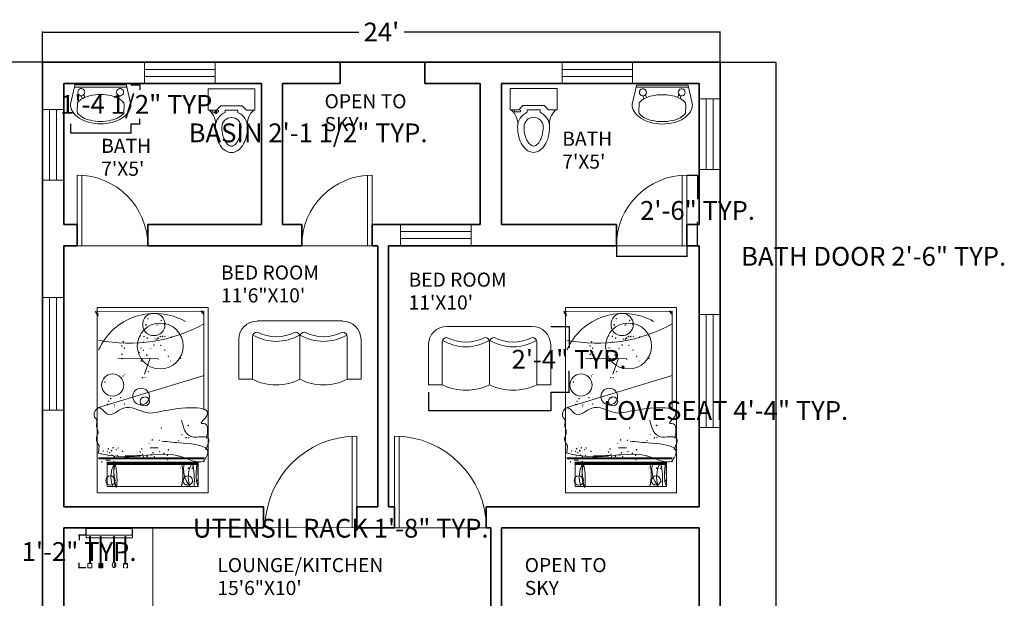
# Model space of a CAD drawing. Units: inches. Extents: x 125 to 976, y 231 to 853.
# Tile 16 of 16: x 557 to 976, y 584 to 830. Entities that reach past the tile are written whole.
import ezdxf

# ---------------------------------------------------------------- set-up
doc = ezdxf.new("R2010")
doc.units = ezdxf.units.IN
doc.header["$MEASUREMENT"] = 0
for name, color, linetype, lineweight in [('A-ANNO-DIMS', 2, 'Continuous', 18), ('A-AREA-IDEN', 7, 'Continuous', 18), ('A-DOOR', 3, 'Continuous', 18), ('A-EQPM', 8, 'Continuous', 15), ('A-FLOR-CASE', 32, 'Continuous', 18), ('A-FLOR-FIXT', 9, 'Continuous', 18), ('A-GLAZ', 4, 'Continuous', 18), ('A-WALL', 7, 'Continuous', 35), ('Furniture', 8, 'Continuous', 15)]:
    doc.layers.add(name, color=color, linetype=linetype, lineweight=lineweight)
doc.styles.get("Standard").update_dxf_attribs({"font": 'italic8.shx'})
doc.dimstyles.get("Standard").update_dxf_attribs({"dimtxt": 8, "dimasz": 0.18, "dimexe": 0.18, "dimexo": 0.0625, "dimgap": 0.09, "dimtad": 0, "dimtih": 1, "dimtoh": 1, "dimdec": 4, "dimzin": 0, "dimdsep": 46, "dimlunit": 3, "dimtxsty": 'Standard', "dimcen": 0.09, "dimclrt": 4, "dimadec": 0, "dimazin": 0, "dimtfac": 1, "dimtdec": 4, "dimtofl": 0, "dimtmove": 0, "dimatfit": 3, "dimfxl": 1, "dimtolj": 1, "dimtzin": 0, "dimarcsym": 0})

# ---------------------------------------------------------------- blocks, each defined once
blk = doc.blocks.new('*D5')
at = {"layer": 'A-ANNO-DIMS', "color": 0, "lineweight": -2, "transparency": 16777216}
for p, q in [((567.19, 812.17), (567.19, 825.16)), ((567.37, 824.98), (701.58, 824.98)), ((855.01, 824.98), (720.81, 824.98)), ((855.19, 812.17), (855.19, 825.16))]:
    blk.add_line(p, q, dxfattribs=at)
at = {"layer": 'A-ANNO-DIMS', "color": 0, "transparency": 16777216}
for points in [[(567.37, 825.01), (567.37, 824.95), (567.19, 824.98)], [(855.01, 825.01), (855.01, 824.95), (855.19, 824.98)]]:
    blk.add_solid(points, dxfattribs=at)
at = {"layer": 'Defpoints', "color": 0, "transparency": 16777216}
for p in [(855.19, 824.98), (567.19, 812.1), (855.19, 812.1)]:
    blk.add_point(p, dxfattribs=at)
at = {"layer": 'A-ANNO-DIMS', "color": 0, "transparency": 16777216, "insert": (711.19, 824.98), "char_height": 8, "attachment_point": 5}
blk.add_mtext("\\A1;24'", dxfattribs=at)
blk = doc.blocks.new('*D6')
at = {"layer": 'A-ANNO-DIMS', "color": 0, "lineweight": -2, "transparency": 16777216}
for p, q in [((855.26, 812.1), (878.96, 812.1)), ((878.78, 811.92), (878.78, 546.96)), ((878.78, 272.28), (878.78, 537.25)), ((846.26, 272.1), (878.96, 272.1))]:
    blk.add_line(p, q, dxfattribs=at)
at = {"layer": 'A-ANNO-DIMS', "color": 0, "transparency": 16777216}
for points in [[(878.75, 811.92), (878.81, 811.92), (878.78, 812.1)], [(878.75, 272.28), (878.81, 272.28), (878.78, 272.1)]]:
    blk.add_solid(points, dxfattribs=at)
at = {"layer": 'Defpoints', "color": 0, "transparency": 16777216}
for p in [(855.19, 812.1), (846.19, 272.1), (878.78, 272.1)]:
    blk.add_point(p, dxfattribs=at)
at = {"layer": 'A-ANNO-DIMS', "color": 0, "transparency": 16777216, "insert": (878.78, 542.1), "char_height": 8, "attachment_point": 5}
blk.add_mtext("\\A1;45'", dxfattribs=at)
blk = doc.blocks.new('BED-SINGLE')
for p, q in [((45.57, 77.25), (0.68, 77.02)), ((1.36, 0), (1.36, 78.74)), ((1.36, 78.74), (48.6, 78.74)), ((46.62, 76.32), (45.83, 76.32)), ((46.75, 35.25), (46.75, 77.26)), ((48.6, 78.74), (48.6, 0)), ((46.75, 35.25), (46.75, 75.28)), ((10.09, 57.07), (27.33, 57.29)), ((21.53, 50.36), (23.91, 57.3)), ((46.77, 49.81), (2, 36.21)), ((46.74, 50.11), (46.74, 35.53)), ((2.2, 19.89), (1.98, 16.84)), ((23.9, 19.06), (27.33, 19.06)), ((46.77, 14.92), (2, 14.9)), ((46.77, 14.62), (2, 14.6)), ((46.75, 14.47), (2.3, 14.45)), ((5.12, 13.84), (6.96, 13.84)), ((44.11, 12.79), (5.52, 12.79)), ((44.11, 12.66), (5.52, 12.66)), ((5.56, 2.64), (5.56, 12.97)), ((5.56, 12.97), (44.32, 12.97)), ((44.26, 2.65), (44.11, 12.79)), ((44.32, 12.97), (44.32, 2.64)), ((44.11, 12.36), (5.52, 12.36)), ((44.11, 12.07), (5.52, 12.07)), ((44.32, 2.64), (5.56, 2.64)), ((1.36, 0), (48.6, 0))]:
    blk.add_line(p, q)
for centre, radius in [((25.44, 71.55), 4.72), ((28.17, 62.4), 9.76), ((22.09, 71.4), 0.118), ((22.93, 74.08), 0.0787), ((26.78, 71.35), 0.118), ((27.34, 71.86), 0.0394), ((28.65, 73.29), 0.118), ((30.02, 71.69), 0.118), ((12.45, 64.21), 0.118), ((19.72, 66.71), 0.118), ((21.26, 66.47), 0.118), ((21.3, 64.04), 0.0787), ((22.64, 65.78), 0.118), ((25.46, 62.84), 0.118), ((25.97, 65.38), 0.0394), ((26.83, 65.34), 0.118), ((27.33, 65.73), 0.118), ((28.16, 66.42), 0.118), ((29.11, 66.45), 0.118), ((30.23, 66.51), 0.0787), ((32.84, 66.14), 0.118), ((11.89, 62.39), 0.118), ((11.89, 58.82), 0.118), ((12.91, 61.47), 0.118), ((19.37, 59.72), 0.0787), ((19.93, 61.53), 0.0787), ((22.48, 58.54), 0.118), ((24.15, 61.41), 0.0394), ((28.4, 62.67), 0.0787), ((30.08, 60.69), 0.118), ((12.09, 56.97), 0.0787), ((20.18, 56), 0.118), ((27.41, 56.76), 0.0394), ((31.66, 58.02), 0.0787), ((32.59, 55.94), 0.0394), ((36.84, 57.2), 0.0787), ((7.95, 45.79), 4.72), ((12.97, 50.24), 0.0394), ((23.12, 51.5), 0.0787), ((4.72, 47.06), 0.118), ((12.36, 49.61), 0.0787), ((20.64, 48.94), 0.118), ((21.75, 49), 0.0787), ((20, 40.91), 3.54), ((5.78, 37.54), 0.118), ((6.3, 38.84), 0.0787), ((7.15, 40.05), 0.118), ((11.34, 40.44), 0.118), ((12.92, 37.77), 0.0787), ((21.58, 38.87), 1.97), ((8.67, 36.51), 0.0394), ((8.72, 37.38), 0.0787), ((19.76, 37.58), 0.0394), ((28.63, 27.54), 0.0787), ((38.69, 26.11), 0.118), ((40.06, 28.61), 0.118), ((23.46, 21.04), 0.0394), ((24.77, 22.46), 0.118), ((27.72, 22.29), 0.0787), ((36.01, 22.18), 0.0394), ((37.38, 24.68), 0.0394), ((39.15, 23.37), 0.118), ((40.26, 23.43), 0.0787), ((3.99, 17.75), 0.118), ((5.75, 17.64), 0.0787), ((6.1, 18.69), 0.118), ((6.65, 17.04), 0.118), ((7.26, 18.11), 0.0394), ((7.48, 17.87), 0.118), ((8.13, 19.13), 0.118), ((9.51, 18.3), 0.118), ((10.16, 19), 0.0787), ((12.17, 17.6), 0.118), ((19.68, 17.32), 0.118), ((20.33, 18.58), 0.118), ((25.12, 17), 0.118), ((27.92, 17.51), 0.0787), ((29.81, 16.72), 0.118), ((31.59, 18.26), 0.118), ((3.44, 13.12), 0.118), ((5.89, 15.61), 0.0394), ((7.14, 14.65), 0.0394), ((7.68, 16.02), 0.0787), ((8.57, 13.26), 0.118), ((8.58, 15.39), 0.118), ((9.94, 15.76), 0.118), ((11.85, 14.52), 0.118), ((19.22, 16.39), 0.0394), ((20.71, 16.3), 0.0787), ((22.61, 15.56), 0.118), ((24.29, 16.17), 0.118), ((25.67, 15.35), 0.118), ((31.19, 15.9), 0.118), ((31.38, 14.05), 0.0787), ((35.87, 15.62), 0.118), ((36.87, 10.58), 0.0394), ((40.18, 10.43), 0.118), ((41.76, 10.43), 0.118), ((42.23, 11.05), 0.118), ((7.01, 5.19), 1.97), ((37.65, 4.55), 0.0394), ((39.85, 5.18), 1.97), ((41.9, 4.7), 0.0787), ((43.48, 4.7), 0.0787), ((43.95, 5.33), 0.0787), ((37.65, 3.45), 0.0394), ((39.23, 3.45), 0.0394), ((39.7, 4.08), 0.0394)]:
    blk.add_circle(centre, radius)
for centre, radius, start, end in [((1.8, 77.16), 1.13, 187.0311, 279.2977), ((2.15, 76.26), 1.02, 131.9337, 260.5378), ((25.86, 50.2), 26.08, 60.1506, 156.1931), ((44.78, 75.28), 1.97, 0, 90), ((45.57, 76.07), 1.18, 0, 90), ((14.92, 129.11), 65.53, 258.633, 299.0775), ((14.39, 67.77), 52.46, 255.8437, 275.7821), ((19.25, 6.76), 12.01, 149.8072, 199.9256), ((25.9, 7.71), 17.5, 163.1329, 196.7593), ((39.3, 10.2), 30.85, 175.6161, 194.8863), ((-19.02, 5.5), 28.83, 354.7074, 14.6885), ((19.98, 7.67), 17.85, 343.6634, 17.1743), ((49.46, 10.01), 11.36, 165.8396, 220.337), ((52.09, 6.75), 12.01, 149.8072, 199.9256), ((13.83, 5.48), 28.83, 354.7074, 14.6885), ((59.92, 7.95), 16.53, 163.0006, 198.6759)]:
    blk.add_arc(centre, radius, start, end)
for points, knots in [([(47.83, 23.01), (48.39, 26.23), (49.02, 29.87), (44.73, 29.28), (54.44, 37.77), (31.08, 35.83), (22.32, 32.61), (13.25, 38.92), (6.29, 30.55), (2.31, 38.17), (-0.92, 33.01), (1.74, 30.96), (0.68, 28.27), (2.31, 25.67), (0.37, 22.75), (1.58, 20.86), (2.2, 19.89)], [0, 0, 0, 0, 6.608381, 7.436978, 10.160479, 26.82811, 35.651646, 45.441607, 52.697614, 57.347481, 61.162366, 63.231685, 65.951856, 68.505046, 71.545852, 74.730692, 74.730692, 74.730692, 74.730692]), ([(47.57, 18.18), (48.41, 20.34), (50.37, 25.33), (39.55, 21.84), (38.02, 27.69), (37.18, 30.9)], [0, 0, 0, 0, 5.247261, 12.129135, 20.530793, 20.530793, 20.530793, 20.530793]), ([(46.4, 13.16), (47.43, 14.71), (50.88, 19.94), (37.54, 21.11), (31.56, 21.67), (28.88, 21.92)], [0, 0, 0, 0, 4.712342, 15.867179, 24.91455, 24.91455, 24.91455, 24.91455]), ([(13.24, 15.66), (15.6, 15.7), (23.87, 15.87), (34.62, 17.37), (42.93, 12.79), (46.01, 13.25), (47.01, 13.4)], [0, 0, 0, 0, 7.121262, 24.909491, 31.123221, 34.101394, 34.101394, 34.101394, 34.101394])]:
    blk.add_open_spline(points, degree=3, knots=knots)
for p in [(21.03, 60.57), (21.03, 40.49), (21.03, 15.28)]:
    blk.add_point(p)
blk = doc.blocks.new('WC')
for p, q in [((0, 27.17), (19.92, 27.17)), ((0, 27.17), (0, 18.11)), ((19.92, 27.17), (19.92, 18.11)), ((0, 18.11), (3.62, 18.11)), ((1.81, 18.11), (1.81, 17.21)), ((1.81, 17.21), (4.07, 17.21)), ((5.43, 19.92), (3.62, 18.11)), ((4.07, 18.11), (3.62, 18.11)), ((5.43, 19.92), (14.48, 19.92)), ((12.67, 18.11), (7.24, 18.11)), ((7.24, 18.11), (7.24, 17.09)), ((12.67, 18.11), (12.67, 17.09)), ((14.48, 19.92), (16.3, 18.11)), ((19.92, 18.11), (16.3, 18.11))]:
    blk.add_line(p, q)
for centre, radius, start, end in [((-4.9, 11.97), 8.15, 352.2011, 48.911), ((9.96, 10.87), 6.79, 113.5782, 180), ((4.07, 17.66), 0.453, 270, 90), ((9.96, 10.87), 6.79, 0, 66.4218), ((24.82, 11.97), 8.15, 131.089, 187.7989), ((9.96, 10.87), 4.07, 0, 180), ((20.49, 10.87), 17.33, 180, 194.5143), ((20.49, 10.87), 14.61, 180, 194.5142), ((-0.58, 10.87), 14.61, 345.4858, 360), ((-0.58, 10.87), 17.33, 345.4857, 360), ((15.3, 9.52), 11.96, 194.5143, 212.0054), ((15.3, 9.52), 9.24, 194.5143, 212.0054), ((12.02, 7.47), 5.38, 212.0054, 236.4659), ((7.9, 7.47), 5.38, 303.5341, 327.9946), ((4.62, 9.52), 9.24, 327.9946, 345.4857), ((4.62, 9.52), 11.96, 327.9946, 345.4857), ((12.02, 7.47), 8.09, 212.0054, 236.4659), ((9.96, 4.37), 4.36, 236.4659, 270), ((9.96, 4.37), 1.65, 236.466, 270), ((9.96, 4.37), 1.65, 270, 303.534), ((9.96, 4.37), 4.36, 270, 303.5341), ((7.9, 7.47), 8.09, 303.5341, 327.9946)]:
    blk.add_arc(centre, radius, start, end)
blk = doc.blocks.new('BASIN')
for p, q in [((0.01, 8.4), (1.8, 16.33)), ((1.8, 16.54), (23.8, 16.54)), ((1.8, 16.13), (1.8, 16.54)), ((23.8, 15.65), (1.8, 15.65)), ((3.17, 14), (3.08, 13.48)), ((3.08, 13.48), (3.17, 12.95)), ((3.42, 14.46), (3.17, 14)), ((3.17, 12.95), (3.42, 12.49)), ((3.81, 14.8), (3.42, 14.46)), ((4.29, 14.98), (3.81, 14.8)), ((4.81, 14.98), (4.29, 14.98)), ((5.29, 14.8), (4.81, 14.98)), ((5.68, 14.46), (5.29, 14.8)), ((5.93, 14), (5.68, 14.46)), ((5.68, 12.49), (5.93, 12.95)), ((6.02, 13.48), (5.93, 14)), ((5.93, 12.95), (6.02, 13.48)), ((19.87, 12.63), (19.34, 11.26)), ((19.66, 14), (19.58, 13.48)), ((19.58, 13.48), (19.66, 12.95)), ((19.92, 14.46), (19.66, 14)), ((19.66, 12.95), (19.92, 12.49)), ((20.31, 14.8), (19.92, 14.46)), ((20.79, 14.98), (20.31, 14.8)), ((21.3, 14.98), (20.79, 14.98)), ((21.79, 14.8), (21.3, 14.98)), ((22.18, 14.46), (21.79, 14.8)), ((22.43, 14), (22.18, 14.46)), ((22.18, 12.49), (22.43, 12.95)), ((22.52, 13.48), (22.43, 14)), ((22.43, 12.95), (22.52, 13.48)), ((23.8, 16.54), (23.8, 16.13)), ((25.59, 8.23), (23.8, 16.33)), ((2.96, 8.83), (2.87, 5.21)), ((2.97, 8.99), (2.96, 8.98)), ((2.96, 8.98), (2.96, 8.97)), ((2.96, 8.97), (2.96, 8.96)), ((2.96, 8.83), (2.96, 8.96)), ((3.07, 9.08), (2.97, 8.99)), ((3.42, 12.49), (3.81, 12.15)), ((3.81, 12.15), (4.29, 11.97)), ((4.29, 11.97), (4.81, 11.97)), ((4.57, 11.96), (5.02, 10.67)), ((4.81, 11.97), (5.29, 12.15)), ((5.29, 12.15), (5.68, 12.49)), ((5.63, 12.45), (6.09, 11.17)), ((19.92, 12.49), (20.31, 12.15)), ((20.31, 12.15), (20.79, 11.97)), ((20.73, 11.97), (20.41, 10.75)), ((20.79, 11.97), (21.3, 11.97)), ((21.3, 11.97), (21.79, 12.15)), ((21.79, 12.15), (22.18, 12.49)), ((22.76, 8.08), (22.65, 8.8)), ((2.87, 5.21), (3, 4.47)), ((3.05, 4.25), (3.05, 4.25)), ((22.54, 4.2), (22.57, 4.35)), ((22.6, 4.46), (22.76, 8.08))]:
    blk.add_line(p, q)
for centre, radius, start, end in [((5.18, 8.21), 5.18, 177.9266, 179.8113), ((8.91, 3.9), 7.83, 118.2302, 139.6822), ((11.35, -0.82), 13.14, 102.6999, 117.8694), ((12.88, -8.38), 20.85, 90.2298, 102.2344), ((12.72, -8.38), 20.85, 77.7656, 89.7702), ((14.25, -0.82), 13.14, 62.1306, 77.3001), ((16.68, 3.89), 7.83, 39.3299, 61.7657), ((5.16, 8.15), 5.16, 179.1785, 213.1413), ((8.98, 10.54), 9.66, 212.6461, 237.0936), ((8.91, 9.59), 7.83, 220.8964, 241.7723), ((16.69, 9.59), 7.83, 298.2281, 319.1983), ((16.64, 10.51), 9.66, 302.4413, 326.8887), ((20.44, 8.09), 5.16, 326.4084, 0.3713), ((20.42, 8.14), 5.18, 359.7541, 0.9471), ((11.42, 14.45), 14.27, 237.383, 254.6821), ((11.35, 14.31), 13.14, 242.1306, 257.3001), ((12.95, 20.75), 20.75, 255.1956, 269.4863), ((12.88, 21.87), 20.85, 257.7656, 269.7702), ((12.76, 20.75), 20.75, 270.0316, 284.3223), ((12.72, 21.87), 20.85, 270.2298, 282.2344), ((14.25, 14.31), 13.14, 282.6999, 297.8694), ((14.23, 14.44), 14.27, 284.841, 302.14)]:
    blk.add_arc(centre, radius, start, end)
blk = doc.blocks.new('UTENSIL-RACK')
for p, q in [((0, 12.76), (0, 13.9)), ((0, 13.9), (19.77, 13.9)), ((19.77, 12.76), (0, 12.76)), ((1.43, 13.28), (1.84, 13.28)), ((1.43, 1.9), (1.43, 13.28)), ((1.84, 13.28), (1.84, 1.9)), ((6.07, 13.28), (6.49, 13.28)), ((6.07, 1.9), (6.07, 13.28)), ((6.49, 13.28), (6.49, 1.9)), ((11.72, 13.28), (12.14, 13.28)), ((11.72, 2.39), (11.72, 13.28)), ((12.14, 13.28), (12.14, 2.38)), ((16.55, 13.28), (16.96, 13.28)), ((16.55, 1.9), (16.55, 13.28)), ((16.96, 13.28), (16.96, 1.9)), ((19.77, 13.9), (19.77, 12.76)), ((0.8, 1.9), (2.53, 1.9)), ((0.8, 0), (0.8, 1.9)), ((2.53, 0), (0.8, 0)), ((1.84, 1.9), (1.43, 1.9)), ((2.53, 1.9), (2.53, 0)), ((5.45, 0), (5.45, 1.9)), ((5.45, 1.9), (7.18, 1.9)), ((5.45, 0), (7.18, 0)), ((5.66, 1.9), (5.73, 1.9)), ((5.66, 0), (5.66, 1.9)), ((5.73, 0), (5.66, 0)), ((5.73, 1.9), (5.73, 0)), ((5.87, 1.89), (5.94, 1.89)), ((5.87, 0), (5.87, 1.89)), ((5.94, 0), (5.87, 0)), ((5.94, 1.89), (5.94, 0)), ((6.49, 1.9), (6.07, 1.9)), ((6.08, 1.9), (6.16, 1.9)), ((6.08, 0), (6.08, 1.9)), ((6.16, 0), (6.08, 0)), ((6.16, 1.9), (6.16, 0)), ((6.29, 1.89), (6.36, 1.89)), ((6.29, 0), (6.29, 1.89)), ((6.36, 0), (6.29, 0)), ((6.36, 1.89), (6.36, 0)), ((6.53, 1.89), (6.6, 1.89)), ((6.53, 0), (6.53, 1.89)), ((6.6, 0), (6.53, 0)), ((6.6, 1.89), (6.6, 0)), ((6.75, 1.9), (6.82, 1.9)), ((6.75, 0), (6.75, 1.9)), ((6.82, 0.01), (6.75, 0)), ((7.18, 0), (6.8, 0)), ((6.82, 1.9), (6.82, 0.01)), ((6.95, 1.89), (7.02, 1.89)), ((6.95, 0), (6.95, 1.89)), ((7.02, 0), (6.95, 0)), ((7.02, 1.89), (7.02, 0)), ((7.18, 1.9), (7.18, 0)), ((15.92, 1.9), (17.65, 1.9)), ((15.92, 0), (15.92, 1.9)), ((16.26, 0.04), (15.92, 0)), ((16.96, 1.9), (16.55, 1.9)), ((17.65, 0), (17.27, 0)), ((17.65, 1.9), (17.65, 0))]:
    blk.add_line(p, q)
for centre, radius, start, end in [((11.03, 1.35), 1.16, 319.28, 30.314), ((16.97, 0.83), 1.06, 115.5387, 227.9153), ((16.58, 0.82), 1.07, 310.1299, 68.3923)]:
    blk.add_arc(centre, radius, start, end)
blk.add_ellipse((11.91, 1.26), major_axis=(0, 1.16), ratio=0.658977)
blk = doc.blocks.new('LOVESEAT')
for p, q in [((44.1, 27.17, -27), (7.88, 27.17, -27)), ((0, 19.29, -27), (0, 2.36, -27)), ((5.91, 20.47, -27), (5.91, 2.36, -27)), ((5.91, 2.36, -27), (5.91, 20.47, -27)), ((5.91, 20.47, -27), (5.91, 2.36, -27)), ((25.99, 2.36, -27), (25.99, 20.47, -27)), ((25.99, 20.47, -27), (25.99, 2.36, -27)), ((46.07, 20.47, -27), (46.07, 2.36, -27)), ((51.97, 2.36, -27), (51.97, 19.29, -27)), ((0, 2.36, -27), (5.91, 2.36, -27)), ((51.97, 2.36, -27), (46.07, 2.36, -27))]:
    blk.add_line(p, q)
for centre, radius, start, end in [((7.88, 19.29, -27), 7.87, 90, 180), ((44.1, 19.29, -27), 7.87, 0, 90), ((7.88, 20.47, -27), 1.97, 90, 180), ((15.95, 38, -27), 19.5, 239.4911, 300.5089), ((15.95, 38, -27), 17.53, 242.5861, 297.4139), ((24.02, 20.47, -27), 1.97, 0, 90), ((27.96, 20.47, -27), 1.97, 90, 180), ((36.03, 38, -27), 19.5, 239.4911, 300.5089), ((36.03, 38, -27), 17.53, 242.5861, 297.4139), ((44.1, 20.47, -27), 1.97, 0, 90), ((15.95, 22.51, -27), 22.51, 243.519, 296.481), ((36.03, 22.51, -27), 22.51, 243.519, 296.481)]:
    blk.add_arc(centre, radius, start, end)
blk = doc.blocks.new('WINDOW-48IN')
for p, q in [((0, 0), (0, 48)), ((0, 48), (9, 48)), ((3, 0), (3, 48)), ((6, 0), (6, 48)), ((9, 48), (9, 0)), ((9, 0), (0, 0))]:
    blk.add_line(p, q)
blk = doc.blocks.new('WINDOW-30IN')
for p, q in [((0, 0), (0, 9)), ((0, 9), (30, 9)), ((30, 9), (30, 0)), ((30, 6), (0, 6)), ((30, 3), (0, 3)), ((30, 0), (0, 0))]:
    blk.add_line(p, q)
blk = doc.blocks.new('DOOR-39IN-LH')
for p, q in [((-2, 0), (-2, 38.95)), ((0, 0), (0, 39)), ((-39, 0.34), (0, 0))]:
    blk.add_line(p, q)
blk.add_arc((0, 0), 39, 90, 179.5065)
blk = doc.blocks.new('DOOR-39IN-RH')
for p, q in [((0, 39), (0, 0)), ((2, 38.95), (2, 0)), ((0, 0), (39, 0))]:
    blk.add_line(p, q)
blk.add_arc((0, 0), 39, 0, 90)
blk = doc.blocks.new('DOOR-30IN')
for p, q in [((-2, 29.93), (-2, 0)), ((0, 30), (0, 0)), ((0, 0), (-30, 0))]:
    blk.add_line(p, q)
blk.add_arc((0, 0), 30, 90, 180)
blk = doc.blocks.new('*D28')
at = {"layer": 'A-ANNO-DIMS', "color": 0, "lineweight": -2, "transparency": 16777216}
for p, q in [((811.01, 734.04), (811.01, 729.42)), ((841.01, 734.04), (841.01, 729.42)), ((811.19, 729.6), (840.83, 729.6)), ((841.01, 729.6), (841.19, 729.6))]:
    blk.add_line(p, q, dxfattribs=at)
at = {"layer": 'A-ANNO-DIMS', "color": 0, "transparency": 16777216}
for points in [[(811.19, 729.63), (811.19, 729.57), (811.01, 729.6)], [(840.83, 729.63), (840.83, 729.57), (841.01, 729.6)]]:
    blk.add_solid(points, dxfattribs=at)
at = {"layer": 'Defpoints', "color": 0, "transparency": 16777216}
for p in [(811.01, 734.1), (841.01, 734.1), (841.01, 729.6)]:
    blk.add_point(p, dxfattribs=at)
at = {"layer": 'A-ANNO-DIMS', "color": 4, "transparency": 16777216, "insert": (920.33, 729.6), "char_height": 8, "attachment_point": 5}
blk.add_mtext('\\A1;BATH DOOR 2\'-6" TYP.', dxfattribs=at)
blk = doc.blocks.new('*D29')
at = {"layer": 'A-ANNO-DIMS', "color": 0, "lineweight": -2, "transparency": 16777216}
for p, q in [((841.07, 764.1), (845.69, 764.1)), ((845.51, 763.92), (845.51, 753.96)), ((845.51, 734.28), (845.51, 744.25)), ((841.07, 734.1), (845.69, 734.1))]:
    blk.add_line(p, q, dxfattribs=at)
at = {"layer": 'A-ANNO-DIMS', "color": 0, "transparency": 16777216}
for points in [[(845.48, 763.92), (845.54, 763.92), (845.51, 764.1)], [(845.48, 734.28), (845.54, 734.28), (845.51, 734.1)]]:
    blk.add_solid(points, dxfattribs=at)
at = {"layer": 'Defpoints', "color": 0, "transparency": 16777216}
for p in [(841.01, 764.1), (845.51, 764.1), (841.01, 734.1)]:
    blk.add_point(p, dxfattribs=at)
at = {"layer": 'A-ANNO-DIMS', "color": 4, "transparency": 16777216, "insert": (845.51, 749.1), "char_height": 8, "attachment_point": 5}
blk.add_mtext('\\A1;2\'-6" TYP.', dxfattribs=at)
blk = doc.blocks.new('*D34')
at = {"layer": 'A-ANNO-DIMS', "color": 0, "lineweight": -2, "transparency": 16777216}
for p, q in [((579.1, 785.87), (579.1, 781.91)), ((604.71, 785.87), (604.71, 781.91)), ((579.28, 782.09), (604.53, 782.09)), ((604.71, 782.09), (604.89, 782.09))]:
    blk.add_line(p, q, dxfattribs=at)
at = {"layer": 'A-ANNO-DIMS', "color": 0, "transparency": 16777216}
for points in [[(579.28, 782.12), (579.28, 782.06), (579.1, 782.09)], [(604.53, 782.12), (604.53, 782.06), (604.71, 782.09)]]:
    blk.add_solid(points, dxfattribs=at)
at = {"layer": 'Defpoints', "color": 0, "transparency": 16777216}
for p in [(579.1, 785.93), (604.71, 785.93), (604.71, 782.09)]:
    blk.add_point(p, dxfattribs=at)
at = {"layer": 'A-ANNO-DIMS', "color": 4, "transparency": 16777216, "insert": (680.03, 782.09), "char_height": 8, "attachment_point": 5}
blk.add_mtext('\\A1;BASIN 2\'-1 1/2" TYP.', dxfattribs=at)
blk = doc.blocks.new('*D35')
at = {"layer": 'A-ANNO-DIMS', "color": 0, "lineweight": -2, "transparency": 16777216}
for p, q in [((604.77, 802.47), (608.73, 802.47)), ((608.55, 802.29), (608.55, 800.39)), ((608.55, 786.11), (608.55, 788.02)), ((604.77, 785.93), (608.73, 785.93))]:
    blk.add_line(p, q, dxfattribs=at)
at = {"layer": 'A-ANNO-DIMS', "color": 0, "transparency": 16777216}
for points in [[(608.52, 802.29), (608.58, 802.29), (608.55, 802.47)], [(608.52, 786.11), (608.58, 786.11), (608.55, 785.93)]]:
    blk.add_solid(points, dxfattribs=at)
at = {"layer": 'Defpoints', "color": 0, "transparency": 16777216}
for p in [(604.71, 802.47), (608.55, 802.47), (604.71, 785.93)]:
    blk.add_point(p, dxfattribs=at)
at = {"layer": 'A-ANNO-DIMS', "color": 4, "transparency": 16777216, "insert": (608.55, 794.2), "char_height": 8, "attachment_point": 5}
blk.add_mtext('\\A1;1\'-4 1/2" TYP.', dxfattribs=at)
blk = doc.blocks.new('*D36')
at = {"layer": 'A-ANNO-DIMS', "color": 0, "lineweight": -2, "transparency": 16777216}
for p, q in [((731.14, 671.77), (731.14, 663.86)), ((783.11, 671.77), (783.11, 663.86)), ((731.32, 664.04), (782.93, 664.04)), ((783.11, 664.04), (783.29, 664.04))]:
    blk.add_line(p, q, dxfattribs=at)
at = {"layer": 'A-ANNO-DIMS', "color": 0, "transparency": 16777216}
for points in [[(731.32, 664.07), (731.32, 664.01), (731.14, 664.04)], [(782.93, 664.07), (782.93, 664.01), (783.11, 664.04)]]:
    blk.add_solid(points, dxfattribs=at)
at = {"layer": 'Defpoints', "color": 0, "transparency": 16777216}
for p in [(731.14, 671.83), (783.11, 671.83), (783.11, 664.04)]:
    blk.add_point(p, dxfattribs=at)
at = {"layer": 'A-ANNO-DIMS', "color": 4, "transparency": 16777216, "insert": (857.48, 664.04), "char_height": 8, "attachment_point": 5}
blk.add_mtext('\\A1;LOVESEAT 4\'-4" TYP.', dxfattribs=at)
blk = doc.blocks.new('*D37')
at = {"layer": 'A-ANNO-DIMS', "color": 0, "lineweight": -2, "transparency": 16777216}
for p, q in [((783.17, 699.78), (791.09, 699.78)), ((790.91, 699.6), (790.91, 690.66)), ((790.91, 672.01), (790.91, 680.96)), ((783.17, 671.83), (791.09, 671.83))]:
    blk.add_line(p, q, dxfattribs=at)
at = {"layer": 'A-ANNO-DIMS', "color": 0, "transparency": 16777216}
for points in [[(790.88, 699.6), (790.94, 699.6), (790.91, 699.78)], [(790.88, 672.01), (790.94, 672.01), (790.91, 671.83)]]:
    blk.add_solid(points, dxfattribs=at)
at = {"layer": 'Defpoints', "color": 0, "transparency": 16777216}
for p in [(783.11, 699.78), (790.91, 699.78), (783.11, 671.83)]:
    blk.add_point(p, dxfattribs=at)
at = {"layer": 'A-ANNO-DIMS', "color": 4, "transparency": 16777216, "insert": (790.91, 685.81), "char_height": 8, "attachment_point": 5}
blk.add_mtext('\\A1;2\'-4" TYP.', dxfattribs=at)
blk = doc.blocks.new('*D52')
at = {"layer": 'A-ANNO-DIMS', "color": 0, "lineweight": -2, "transparency": 16777216}
for p, q in [((585.68, 611.05), (585.68, 614.14)), ((585.86, 613.96), (605.27, 613.96)), ((605.45, 611.05), (605.45, 614.14)), ((605.45, 613.96), (605.63, 613.96))]:
    blk.add_line(p, q, dxfattribs=at)
at = {"layer": 'A-ANNO-DIMS', "color": 0, "transparency": 16777216}
for points in [[(585.86, 613.99), (585.86, 613.93), (585.68, 613.96)], [(605.27, 613.99), (605.27, 613.93), (605.45, 613.96)]]:
    blk.add_solid(points, dxfattribs=at)
at = {"layer": 'Defpoints', "color": 0, "transparency": 16777216}
for p in [(585.68, 610.99), (605.45, 613.96), (605.45, 610.99)]:
    blk.add_point(p, dxfattribs=at)
at = {"layer": 'A-ANNO-DIMS', "color": 4, "transparency": 16777216, "insert": (693.91, 613.96), "char_height": 8, "attachment_point": 5}
blk.add_mtext('\\A1;UTENSIL RACK 1\'-8" TYP.', dxfattribs=at)
blk = doc.blocks.new('*D53')
at = {"layer": 'A-ANNO-DIMS', "color": 0, "lineweight": -2, "transparency": 16777216}
for p, q in [((585.62, 610.99), (582.54, 610.99)), ((582.72, 610.81), (582.72, 608.9)), ((582.72, 597.28), (582.72, 599.19)), ((585.62, 597.1), (582.54, 597.1))]:
    blk.add_line(p, q, dxfattribs=at)
at = {"layer": 'A-ANNO-DIMS', "color": 0, "transparency": 16777216}
for points in [[(582.69, 610.81), (582.75, 610.81), (582.72, 610.99)], [(582.69, 597.28), (582.75, 597.28), (582.72, 597.1)]]:
    blk.add_solid(points, dxfattribs=at)
at = {"layer": 'Defpoints', "color": 0, "transparency": 16777216}
for p in [(582.72, 610.99), (585.68, 610.99), (585.68, 597.1)]:
    blk.add_point(p, dxfattribs=at)
at = {"layer": 'A-ANNO-DIMS', "color": 4, "transparency": 16777216, "insert": (582.72, 604.04), "char_height": 8, "attachment_point": 5}
blk.add_mtext('\\A1;1\'-2" TYP.', dxfattribs=at)
blk = doc.blocks.new('*D57')
at = {"layer": 'A-ANNO-DIMS', "color": 0, "lineweight": -2, "transparency": 16777216}
for p, q in [((567.13, 812.1), (538.31, 812.1)), ((538.49, 811.92), (538.49, 575.46)), ((538.49, 329.28), (538.49, 565.75)), ((576.13, 329.1), (538.31, 329.1))]:
    blk.add_line(p, q, dxfattribs=at)
at = {"layer": 'A-ANNO-DIMS', "color": 0, "transparency": 16777216}
for points in [[(538.46, 811.92), (538.52, 811.92), (538.49, 812.1)], [(538.46, 329.28), (538.52, 329.28), (538.49, 329.1)]]:
    blk.add_solid(points, dxfattribs=at)
at = {"layer": 'Defpoints', "color": 0, "transparency": 16777216}
for p in [(538.49, 812.1), (567.19, 812.1), (576.19, 329.1)]:
    blk.add_point(p, dxfattribs=at)
at = {"layer": 'A-ANNO-DIMS', "color": 4, "transparency": 16777216, "insert": (538.49, 570.6), "char_height": 8, "attachment_point": 5}
blk.add_mtext('\\A1;40\'-3"', dxfattribs=at)

msp = doc.modelspace()

# ---------------------------------------------------------------- linework, layer by layer
at = {"layer": 'A-FLOR-CASE'}
msp.add_line((614.10131, 536.20453), (614.10131, 614.10475), dxfattribs=at)
at = {"layer": 'A-WALL'}
for p, q in [((693.64668, 803.10475), (693.64668, 812.10475)), ((729.64668, 803.10475), (729.64668, 812.10475)), ((576.19287, 803.10475), (660.19287, 803.10475)), ((576.19287, 743.10475), (576.19287, 803.10475)), ((660.19287, 743.10475), (660.19287, 803.10475)), ((669.19287, 743.10475), (669.19287, 803.10475)), ((669.19287, 803.10475), (693.64668, 803.10475)), ((729.64668, 803.10475), (753.19287, 803.10475)), ((753.19287, 803.10475), (753.19287, 743.10475)), ((762.19287, 803.10475), (762.19287, 743.10475)), ((762.19287, 803.10475), (846.19287, 803.10475)), ((846.19287, 803.10475), (846.19287, 743.10475)), ((576.19287, 743.10475), (581.94156, 743.10475)), ((581.94156, 743.10475), (581.94156, 734.10475)), ((611.94156, 743.10475), (611.94156, 734.10475)), ((611.94156, 743.10475), (660.19287, 743.10475)), ((669.19287, 743.10475), (677.32566, 743.10475)), ((677.32566, 734.10475), (677.32566, 743.10475)), ((707.32566, 734.10475), (707.32566, 743.10475)), ((707.32566, 743.10475), (753.19287, 743.10475)), ((762.19287, 743.10475), (811.00974, 743.10475)), ((811.00974, 743.10475), (811.00974, 734.10475)), ((841.00974, 743.10475), (841.00974, 734.10475)), ((841.00974, 743.10475), (846.19287, 743.10475)), ((576.19287, 734.10475), (581.94156, 734.10475)), ((576.19287, 623.10475), (576.19287, 734.10475)), ((611.94156, 734.10475), (677.32566, 734.10475)), ((707.32566, 734.10475), (709.69287, 734.10475)), ((709.69287, 734.10475), (709.69287, 623.10475)), ((714.19287, 734.10475), (714.19287, 623.10475)), ((714.19287, 734.10475), (811.00974, 734.10475)), ((841.00974, 734.10475), (846.19287, 734.10475)), ((846.19287, 734.10475), (846.19287, 623.10475)), ((661.15418, 623.10475), (576.19287, 623.10475)), ((661.15418, 614.10475), (661.15418, 623.10475)), ((700.75418, 614.10475), (700.75418, 623.10475)), ((709.69287, 623.10475), (700.75418, 623.10475)), ((716.71926, 623.10475), (714.19287, 623.10475)), ((716.71926, 614.10475), (716.71926, 623.10475)), ((846.19287, 623.10475), (755.71926, 623.10475)), ((755.71926, 614.10475), (755.71926, 623.10475)), ((576.19287, 614.10475), (661.15418, 614.10475)), ((576.19287, 503.10475), (576.19287, 614.10475)), ((700.75418, 614.10475), (716.71926, 614.10475)), ((755.71926, 614.10475), (757.69287, 614.10475)), ((757.69287, 503.10475), (757.69287, 614.10475)), ((762.19287, 503.10475), (762.19287, 614.10475)), ((762.19287, 614.10475), (846.19287, 614.10475)), ((846.19287, 614.10475), (846.19287, 503.10475))]:
    msp.add_line(p, q, dxfattribs=at)
msp.add_lwpolyline([(567.19287, 812.10475), (855.19287, 812.10475), (855.19287, 272.10475), (567.19287, 272.10475)], close=True, dxfattribs=at)

# ---------------------------------------------------------------- block references
at = {"layer": 'A-DOOR', "extrusion": (0, 0, -1), "zscale": -1}
msp.add_blockref('DOOR-30IN', (-581.94156, 734.10475), dxfattribs=at)
at = {"layer": 'A-DOOR'}
for name, p in [('DOOR-30IN', (707.32566, 734.10475)), ('DOOR-30IN', (841.00974, 734.10475)), ('DOOR-39IN-LH', (700.75418, 614.10475)), ('DOOR-39IN-RH', (716.71926, 614.10475))]:
    msp.add_blockref(name, p, dxfattribs=at)
at = {"layer": 'A-EQPM'}
msp.add_blockref('UTENSIL-RACK', (585.68011, 597.09443), dxfattribs=at)
at = {"layer": 'A-FLOR-FIXT'}
for name, p in [('BASIN', (579.10998, 785.93398)), ('WC', (637.5139, 773.68603)), ('WC', (765.9035, 773.75878)), ('BASIN', (817.74166, 785.84871))]:
    msp.add_blockref(name, p, dxfattribs=at)
at = {"layer": 'A-GLAZ'}
for name, p in [('WINDOW-30IN', (610.48384, 803.1)), ('WINDOW-30IN', (787.94, 803.1)), ('WINDOW-30IN', (719.28301, 734.1)), ('WINDOW-48IN', (567.19, 664.10591)), ('WINDOW-48IN', (846.19, 656.84411))]:
    msp.add_blockref(name, p, dxfattribs=at)
at = {"layer": 'A-GLAZ', "rotation": 269.9999999999997}
for p in [(846.18812, 796.55668), (567.18812, 792.00243)]:
    msp.add_blockref('WINDOW-30IN', p, dxfattribs=at)
at = {"layer": 'Furniture'}
for name, p in [('BED-SINGLE', (589.04801, 629.05)), ('BED-SINGLE', (788.02432, 629.05)), ('LOVESEAT', (650.56, 674.92)), ('LOVESEAT', (731.14079, 672.61959))]:
    msp.add_blockref(name, p, dxfattribs=at)

# ---------------------------------------------------------------- texts
at = {"layer": 'A-AREA-IDEN'}
for s, p in [('OPEN TO ', (687.03793, 792.53471)), ('SKY', (687.03793, 782.82042)), ('BATH', (788.02457, 776.60255)), ('BATH', (592.12556, 773.56788)), ("7'X5'", (592.12556, 763.85359)), ("7'X5'", (788.02457, 766.88827)), ('BED ROOM', (642.99861, 719.70206)), ('BED ROOM', (722.72494, 716.66739)), ('11\'6"X10\'', (642.99861, 709.98778)), ("11'X10'", (722.72494, 706.95311)), ('LOUNGE/KITCHEN', (641.48004, 595.27965)), ('OPEN TO ', (772.07931, 595.27965)), ('15\'6"X10\'', (641.48004, 585.56536)), ('SKY', (772.07931, 585.56536))]:
    msp.add_text(s, height=6, dxfattribs=at).set_placement(p)

# ---------------------------------------------------------------- dimensions: what is measured, and where the dimension line sits
at = {"layer": 'A-ANNO-DIMS'}
dim = msp.add_linear_dim(base=(855.19287, 824.97552), p1=(567.19287, 812.10475), p2=(855.19287, 812.10475), dimstyle='Standard', override={"dimclrd": 0, "dimclre": 0, "dimclrt": 0}, dxfattribs=at)
dim.commit()
dim.dimension.update_dxf_attribs({"geometry": '*D5', "text_midpoint": (711.19287, 824.97552)})
for base, p1, p2, override, picture, middle in [((538.49287, 812.10475), (576.19287, 329.10475), (567.19287, 812.10475), {"dimdec": 1, "dimlfac": 1, "dimrnd": 0, "dimzin": 1, "dimdsep": 46, "dimlunit": 4, "dimfrac": 2}, '*D57', (538.49287, 570.60475)), ((878.78186, 272.10475), (855.19287, 812.10475), (846.19287, 272.10475), {"dimclrd": 0, "dimclre": 0, "dimclrt": 0}, '*D6', (878.78186, 542.10475))]:
    dim = msp.add_linear_dim(base=base, p1=p1, p2=p2, angle=90, dimstyle='Standard', override=override, dxfattribs=at)
    dim.commit()
    dim.dimension.update_dxf_attribs({"geometry": picture, "text_midpoint": middle})
for base, p1, p2, picture, middle in [((608.55337, 802.47025), (604.71159, 785.93485), (604.71159, 802.47025), '*D35', (608.55337, 794.20255)), ((845.50974, 764.10475), (841.00974, 734.10475), (841.00974, 764.10475), '*D29', (845.50974, 749.10475)), ((790.9076, 699.78488), (783.11234, 671.83218), (783.11234, 699.78488), '*D37', (790.9076, 685.80853)), ((582.71589, 610.99065), (585.6814, 597.09685), (585.6814, 610.99065), '*D53', (582.71589, 604.04375))]:
    dim = msp.add_linear_dim(base=base, p1=p1, p2=p2, angle=90, text='<> TYP.', dimstyle='Standard', override={"dimdec": 1, "dimlfac": 1, "dimrnd": 0, "dimzin": 1, "dimdsep": 46, "dimlunit": 4, "dimfrac": 2}, dxfattribs=at)
    dim.commit()
    dim.dimension.update_dxf_attribs({"geometry": picture, "text_midpoint": middle})
for base, p1, p2, text, picture, middle in [((604.71159, 782.09307), (579.09971, 785.93485), (604.71159, 785.93485), 'BASIN <> TYP.', '*D34', (680.02921, 782.09307)), ((841.00974, 729.60475), (811.00974, 734.10475), (841.00974, 734.10475), 'BATH DOOR <> TYP.', '*D28', (920.32736, 729.60475)), ((783.11234, 664.03692), (731.14394, 671.83218), (783.11234, 671.83218), 'LOVESEAT <> TYP.', '*D36', (857.47758, 664.03692)), ((605.45146, 613.95616), (585.6814, 610.99065), (605.45146, 610.99065), 'UTENSIL RACK <> TYP.', '*D52', (693.91194, 613.95616))]:
    dim = msp.add_linear_dim(base=base, p1=p1, p2=p2, text=text, dimstyle='Standard', override={"dimdec": 1, "dimlfac": 1, "dimrnd": 0, "dimzin": 1, "dimdsep": 46, "dimlunit": 4, "dimfrac": 2}, dxfattribs=at)
    dim.commit()
    dim.dimension.update_dxf_attribs({"geometry": picture, "text_midpoint": middle})

doc.saveas('drawing.dxf')
